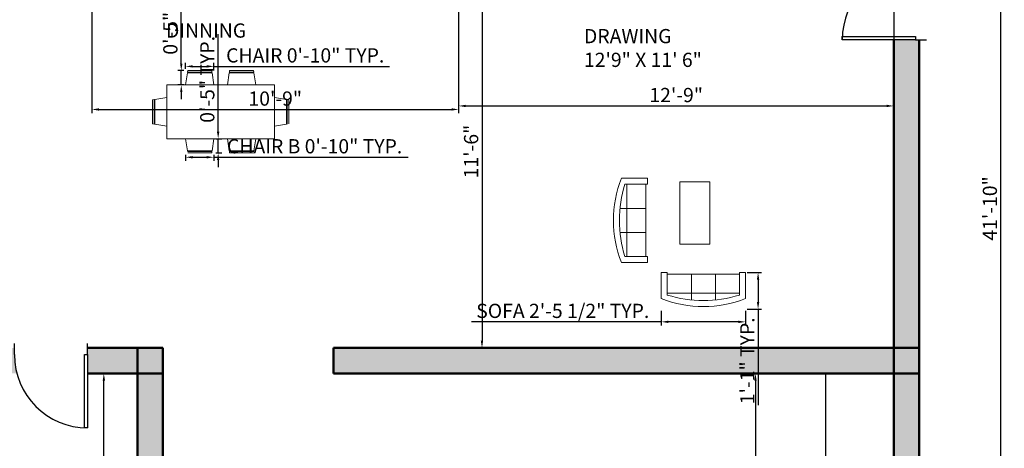
# Model space of a CAD drawing. Units: millimetres. Extents: x 2829 to 4029, y 962 to 1687.
# Tile 3 of 7: x 3053 to 3399, y 1289 to 1440. Entities that reach past the tile are written whole.
import ezdxf

# ---------------------------------------------------------------- set-up
doc = ezdxf.new("R2010")
doc.units = ezdxf.units.MM
for name, color, linetype, lineweight in [('A-ANNO-DIMS', 140, 'Continuous', 18), ('A-AREA-IDEN', 190, 'Continuous', 25), ('A-FLOR-CASE', 90, 'Continuous', 25), ('A-WALL-PATT', 2, 'Continuous', 13), ('doors', 10, 'Continuous', 25), ('furniture', 90, 'Continuous', 18), ('walls', 50, 'Continuous', 50)]:
    doc.layers.add(name, color=color, linetype=linetype, lineweight=lineweight)
doc.styles.get("Standard").update_dxf_attribs({"font": 'arial.ttf'})
doc.dimstyles.new('ISO-25', dxfattribs={"dimtxt": 5, "dimasz": 2.5, "dimexe": 1.25, "dimexo": 0.625, "dimtad": 1, "dimdec": 0, "dimlunit": 3, "dimtxsty": 'Standard', "dimcen": 2.5, "dimadec": 0, "dimazin": 0, "dimtfac": 1, "dimtdec": 0, "dimtmove": 0, "dimatfit": 3, "dimfxl": 1, "dimarcsym": 0})

# ---------------------------------------------------------------- blocks, each defined once
blk = doc.blocks.new('*U2')
for p, q in [((0, 0), (0, -6)), ((40, 0), (40, -6))]:
    blk.add_line(p, q)
blk.add_lwpolyline([(0, 0), (0, 40), (1.75, 40), (1.75, 0)], close=True)
blk.add_arc((0, 0), 40, 0, 90)
blk = doc.blocks.new('Sofa - Roundback 7 ft.')
for p, q in [((-12.00002, -32.4421), (-12.00003, -6.5971)), ((11.99997, -32.4421), (11.99998, -6.5971)), ((-36.000027, -34), (-36.000027, -11.4696)), ((-35.999844, -13.3819), (35.9998, -13.3819)), ((35.99998, -34), (35.99998, -11.4696)), ((-36.000027, -32.4421), (35.99998, -32.4421))]:
    blk.add_line(p, q)
for points in [[(-36.000027, -34), (-42.000027, -34), (-42.000027, -8)], [(41.99998, -8), (41.99998, -34), (35.99998, -34)]]:
    blk.add_lwpolyline(points)
for centre, radius, start, end in [((0, -114.25), 114.25, 68.43141, 111.5686), ((-0.00001, -127.1968), 121.1968, 72.72033, 107.2797)]:
    blk.add_arc(centre, radius, start, end)
blk = doc.blocks.new('*D21')
at = {"layer": 'A-ANNO-DIMS', "color": 0, "lineweight": -2, "transparency": 16777216}
for p, q in [((3080.87, 1315.38), (3083.77, 1315.38)), ((3082.52, 1133.88), (3082.52, 1312.88)), ((3078.75, 1131.38), (3083.77, 1131.38))]:
    blk.add_line(p, q, dxfattribs=at)
at = {"layer": 'A-ANNO-DIMS', "color": 0, "transparency": 16777216}
for points in [[(3082.11, 1312.88), (3082.94, 1312.88), (3082.52, 1315.38)], [(3082.11, 1133.88), (3082.94, 1133.88), (3082.52, 1131.38)]]:
    blk.add_solid(points, dxfattribs=at)
at = {"layer": 'Defpoints', "color": 0, "transparency": 16777216}
for p in [(3080.25, 1315.38), (3082.52, 1315.38), (3078.12, 1131.38)]:
    blk.add_point(p, dxfattribs=at)
at = {"layer": 'A-ANNO-DIMS', "color": 0, "transparency": 16777216, "insert": (3079.34, 1223.38), "char_height": 5, "attachment_point": 5, "rotation": 90}
blk.add_mtext('15\'-4"', dxfattribs=at)
blk = doc.blocks.new('*D25')
at = {"layer": 'A-ANNO-DIMS', "color": 0, "lineweight": -2, "transparency": 16777216}
for p, q in [((3311.7, 1312.88), (3311.7, 1199.88)), ((3312.32, 1315.38), (3312.95, 1315.38)), ((3312.32, 1197.38), (3312.95, 1197.38))]:
    blk.add_line(p, q, dxfattribs=at)
at = {"layer": 'A-ANNO-DIMS', "color": 0, "transparency": 16777216}
for points in [[(3311.28, 1312.88), (3312.11, 1312.88), (3311.7, 1315.38)], [(3311.28, 1199.88), (3312.11, 1199.88), (3311.7, 1197.38)]]:
    blk.add_solid(points, dxfattribs=at)
at = {"layer": 'Defpoints', "color": 0, "transparency": 16777216}
for p in [(3311.7, 1315.38), (3311.7, 1197.38), (3311.7, 1197.38)]:
    blk.add_point(p, dxfattribs=at)
at = {"layer": 'A-ANNO-DIMS', "color": 0, "transparency": 16777216, "insert": (3308.52, 1256.38), "char_height": 5, "attachment_point": 5, "rotation": 90}
blk.add_mtext('9\'-10"', dxfattribs=at)
blk = doc.blocks.new('*D28')
at = {"layer": 'A-ANNO-DIMS', "color": 0, "lineweight": -2, "transparency": 16777216}
for p, q in [((3215.69, 1462.38), (3214.27, 1462.38)), ((3215.52, 1459.88), (3215.52, 1326.88)), ((3215.69, 1324.38), (3214.27, 1324.38))]:
    blk.add_line(p, q, dxfattribs=at)
at = {"layer": 'A-ANNO-DIMS', "color": 0, "transparency": 16777216}
for points in [[(3215.1, 1459.88), (3215.93, 1459.88), (3215.52, 1462.38)], [(3215.1, 1326.88), (3215.93, 1326.88), (3215.52, 1324.38)]]:
    blk.add_solid(points, dxfattribs=at)
at = {"layer": 'Defpoints', "color": 0, "transparency": 16777216}
for p in [(3216.31, 1462.38), (3215.52, 1324.38), (3216.31, 1324.38)]:
    blk.add_point(p, dxfattribs=at)
at = {"layer": 'A-ANNO-DIMS', "color": 0, "transparency": 16777216, "insert": (3212.34, 1393.38), "char_height": 5, "attachment_point": 5, "rotation": 90}
blk.add_mtext('11\'-6"', dxfattribs=at)
blk = doc.blocks.new('*D29')
at = {"layer": 'A-ANNO-DIMS', "color": 0, "lineweight": -2, "transparency": 16777216}
for p, q in [((3207.31, 1461.76), (3207.31, 1408.16)), ((3360.31, 1461.76), (3360.31, 1408.16)), ((3209.81, 1409.41), (3357.81, 1409.41))]:
    blk.add_line(p, q, dxfattribs=at)
at = {"layer": 'A-ANNO-DIMS', "color": 0, "transparency": 16777216}
for points in [[(3209.81, 1409.83), (3209.81, 1408.99), (3207.31, 1409.41)], [(3357.81, 1409.83), (3357.81, 1408.99), (3360.31, 1409.41)]]:
    blk.add_solid(points, dxfattribs=at)
at = {"layer": 'Defpoints', "color": 0, "transparency": 16777216}
for p in [(3207.31, 1462.38), (3360.31, 1462.38), (3360.31, 1409.41)]:
    blk.add_point(p, dxfattribs=at)
at = {"layer": 'A-ANNO-DIMS', "color": 0, "transparency": 16777216, "insert": (3283.81, 1412.59), "char_height": 5, "attachment_point": 5}
blk.add_mtext('12\'-9"', dxfattribs=at)
blk = doc.blocks.new('*D30')
at = {"layer": 'A-ANNO-DIMS', "color": 0, "lineweight": -2, "transparency": 16777216}
for p, q in [((3078.31, 1461.76), (3078.31, 1406.92)), ((3207.31, 1461.76), (3207.31, 1406.92)), ((3080.81, 1408.17), (3204.81, 1408.17))]:
    blk.add_line(p, q, dxfattribs=at)
at = {"layer": 'A-ANNO-DIMS', "color": 0, "transparency": 16777216}
for points in [[(3080.81, 1408.59), (3080.81, 1407.75), (3078.31, 1408.17)], [(3204.81, 1408.59), (3204.81, 1407.75), (3207.31, 1408.17)]]:
    blk.add_solid(points, dxfattribs=at)
at = {"layer": 'Defpoints', "color": 0, "transparency": 16777216}
for p in [(3078.31, 1462.38), (3207.31, 1462.38), (3207.31, 1408.17)]:
    blk.add_point(p, dxfattribs=at)
at = {"layer": 'A-ANNO-DIMS', "color": 0, "transparency": 16777216, "insert": (3142.81, 1411.35), "char_height": 5, "attachment_point": 5}
blk.add_mtext('10\'-9"', dxfattribs=at)
blk = doc.blocks.new('CHAIR-DINING-COMPACT')
for p, q in [((0.66, 4.21), (0, 0)), ((0.66, 4.21), (9.32, 4.21)), ((0.78, 5), (0.7, 4.47)), ((9.28, 4.47), (0.7, 4.47)), ((0.78, 5), (9.2, 5)), ((9.28, 4.47), (9.2, 5)), ((9.98, 0), (9.32, 4.21))]:
    blk.add_line(p, q)
blk = doc.blocks.new('CHAIR-DINING-COMPACT-B')
for p, q in [((0.66, 0.79), (0, 5)), ((9.98, 5), (9.32, 0.79)), ((0.66, 0.79), (9.32, 0.79)), ((9.28, 0.53), (0.7, 0.53)), ((0.78, 0), (9.2, 0)), ((9.28, 0.53), (9.2, 0))]:
    blk.add_line(p, q)
blk = doc.blocks.new('TABLE-COFFEE-RECT')
blk.add_lwpolyline([(0, 0), (10.49, 0), (10.49, 21.96), (0, 21.96)], close=True)
blk = doc.blocks.new('*D65')
at = {"layer": 'A-ANNO-DIMS', "color": 0, "lineweight": -2, "transparency": 16777216}
for p, q in [((3278.58, 1337.35), (3278.58, 1332.28)), ((3308.17, 1337.35), (3308.17, 1332.28)), ((3278.58, 1333.53), (3211.77, 1333.53)), ((3305.67, 1333.53), (3281.08, 1333.53))]:
    blk.add_line(p, q, dxfattribs=at)
at = {"layer": 'A-ANNO-DIMS', "color": 0, "transparency": 16777216}
for points in [[(3281.08, 1333.95), (3281.08, 1333.11), (3278.58, 1333.53)], [(3305.67, 1333.95), (3305.67, 1333.11), (3308.17, 1333.53)]]:
    blk.add_solid(points, dxfattribs=at)
at = {"layer": 'Defpoints', "color": 0, "transparency": 16777216}
for p in [(3278.58, 1337.97), (3308.17, 1337.97), (3278.58, 1333.53)]:
    blk.add_point(p, dxfattribs=at)
at = {"layer": 'A-ANNO-DIMS', "color": 0, "transparency": 16777216, "insert": (3243.92, 1336.74), "char_height": 5, "attachment_point": 5}
blk.add_mtext('SOFA 2\'-5 1/2" TYP.', dxfattribs=at)
blk = doc.blocks.new('*D66')
at = {"layer": 'A-ANNO-DIMS', "color": 0, "lineweight": -2, "transparency": 16777216}
for p, q in [((3308.8, 1350.89), (3313.86, 1350.89)), ((3312.61, 1348.39), (3312.61, 1340.47)), ((3308.8, 1337.97), (3313.86, 1337.97)), ((3312.61, 1337.97), (3312.61, 1304.21))]:
    blk.add_line(p, q, dxfattribs=at)
at = {"layer": 'A-ANNO-DIMS', "color": 0, "transparency": 16777216}
for points in [[(3312.19, 1348.39), (3313.03, 1348.39), (3312.61, 1350.89)], [(3312.19, 1340.47), (3313.03, 1340.47), (3312.61, 1337.97)]]:
    blk.add_solid(points, dxfattribs=at)
at = {"layer": 'Defpoints', "color": 0, "transparency": 16777216}
for p in [(3308.17, 1350.89), (3308.17, 1337.97), (3312.61, 1337.97)]:
    blk.add_point(p, dxfattribs=at)
at = {"layer": 'A-ANNO-DIMS', "color": 0, "transparency": 16777216, "insert": (3309.47, 1319.84), "char_height": 5, "attachment_point": 5, "rotation": 90}
blk.add_mtext('1\'-1" TYP.', dxfattribs=at)
blk = doc.blocks.new('*D79')
at = {"layer": 'A-ANNO-DIMS', "color": 0, "lineweight": -2, "transparency": 16777216}
for p, q in [((3111.25, 1422.43), (3111.25, 1424.56)), ((3113.75, 1423.31), (3118.73, 1423.31)), ((3121.23, 1422.43), (3121.23, 1424.56)), ((3121.23, 1423.31), (3182.96, 1423.31))]:
    blk.add_line(p, q, dxfattribs=at)
at = {"layer": 'A-ANNO-DIMS', "color": 0, "transparency": 16777216}
for points in [[(3113.75, 1423.72), (3113.75, 1422.89), (3111.25, 1423.31)], [(3118.73, 1423.72), (3118.73, 1422.89), (3121.23, 1423.31)]]:
    blk.add_solid(points, dxfattribs=at)
at = {"layer": 'Defpoints', "color": 0, "transparency": 16777216}
for p in [(3121.23, 1423.31), (3111.25, 1421.81), (3121.23, 1421.81)]:
    blk.add_point(p, dxfattribs=at)
at = {"layer": 'A-ANNO-DIMS', "color": 0, "transparency": 16777216, "insert": (3153.35, 1426.52), "char_height": 5, "attachment_point": 5}
blk.add_mtext('CHAIR 0\'-10" TYP.', dxfattribs=at)
blk = doc.blocks.new('*D80')
at = {"layer": 'A-ANNO-DIMS', "color": 0, "lineweight": -2, "transparency": 16777216}
for p, q in [((3109.76, 1424.31), (3109.76, 1458.54)), ((3110.63, 1421.81), (3108.51, 1421.81)), ((3109.76, 1416.81), (3109.76, 1421.81)), ((3110.63, 1416.81), (3108.51, 1416.81)), ((3109.76, 1414.31), (3109.76, 1411.81))]:
    blk.add_line(p, q, dxfattribs=at)
at = {"layer": 'A-ANNO-DIMS', "color": 0, "transparency": 16777216}
for points in [[(3109.34, 1424.31), (3110.17, 1424.31), (3109.76, 1421.81)], [(3109.34, 1414.31), (3110.17, 1414.31), (3109.76, 1416.81)]]:
    blk.add_solid(points, dxfattribs=at)
at = {"layer": 'Defpoints', "color": 0, "transparency": 16777216}
for p in [(3109.76, 1421.81), (3111.25, 1421.81), (3111.25, 1416.81)]:
    blk.add_point(p, dxfattribs=at)
at = {"layer": 'A-ANNO-DIMS', "color": 0, "transparency": 16777216, "insert": (3106.58, 1442.67), "char_height": 5, "attachment_point": 5, "rotation": 90}
blk.add_mtext('0\'-5" TYP.', dxfattribs=at)
blk = doc.blocks.new('*D85')
at = {"layer": 'A-ANNO-DIMS', "color": 0, "lineweight": -2, "transparency": 16777216}
for p, q in [((3111.25, 1392.25), (3111.25, 1390.13)), ((3121.23, 1392.25), (3121.23, 1390.13)), ((3113.75, 1391.38), (3118.73, 1391.38)), ((3121.23, 1391.38), (3189.56, 1391.38))]:
    blk.add_line(p, q, dxfattribs=at)
at = {"layer": 'A-ANNO-DIMS', "color": 0, "transparency": 16777216}
for points in [[(3113.75, 1391.79), (3113.75, 1390.96), (3111.25, 1391.38)], [(3118.73, 1391.79), (3118.73, 1390.96), (3121.23, 1391.38)]]:
    blk.add_solid(points, dxfattribs=at)
at = {"layer": 'Defpoints', "color": 0, "transparency": 16777216}
for p in [(3111.25, 1392.87), (3121.23, 1392.87), (3121.23, 1391.38)]:
    blk.add_point(p, dxfattribs=at)
at = {"layer": 'A-ANNO-DIMS', "color": 0, "transparency": 16777216, "insert": (3156.65, 1394.59), "char_height": 5, "attachment_point": 5}
blk.add_mtext('CHAIR B 0\'-10" TYP.', dxfattribs=at)
blk = doc.blocks.new('*D86')
at = {"layer": 'A-ANNO-DIMS', "color": 0, "lineweight": -2, "transparency": 16777216}
for p, q in [((3122.73, 1400.37), (3122.73, 1434.6)), ((3121.86, 1397.87), (3123.98, 1397.87)), ((3122.73, 1392.87), (3122.73, 1397.87)), ((3121.86, 1392.87), (3123.98, 1392.87)), ((3122.73, 1390.37), (3122.73, 1387.87))]:
    blk.add_line(p, q, dxfattribs=at)
at = {"layer": 'A-ANNO-DIMS', "color": 0, "transparency": 16777216}
for points in [[(3122.31, 1400.37), (3123.15, 1400.37), (3122.73, 1397.87)], [(3122.31, 1390.37), (3123.15, 1390.37), (3122.73, 1392.87)]]:
    blk.add_solid(points, dxfattribs=at)
at = {"layer": 'Defpoints', "color": 0, "transparency": 16777216}
for p in [(3121.23, 1397.87), (3122.73, 1397.87), (3121.23, 1392.87)]:
    blk.add_point(p, dxfattribs=at)
at = {"layer": 'A-ANNO-DIMS', "color": 0, "transparency": 16777216, "insert": (3119.55, 1418.74), "char_height": 5, "attachment_point": 5, "rotation": 90}
blk.add_mtext('0\'-5" TYP.', dxfattribs=at)
blk = doc.blocks.new('*D89')
at = {"layer": 'A-ANNO-DIMS', "color": 0, "lineweight": -2, "transparency": 16777216}
for p, q in [((2853.31, 1314.76), (2853.31, 1094.98)), ((3369.31, 1121.76), (3369.31, 1094.98)), ((2855.81, 1096.23), (3366.81, 1096.23))]:
    blk.add_line(p, q, dxfattribs=at)
at = {"layer": 'A-ANNO-DIMS', "color": 0, "transparency": 16777216}
for points in [[(2855.81, 1096.65), (2855.81, 1095.81), (2853.31, 1096.23)], [(3366.81, 1096.65), (3366.81, 1095.81), (3369.31, 1096.23)]]:
    blk.add_solid(points, dxfattribs=at)
at = {"layer": 'Defpoints', "color": 0, "transparency": 16777216}
for p in [(2853.31, 1315.38), (3369.31, 1122.38), (3369.31, 1096.23)]:
    blk.add_point(p, dxfattribs=at)
at = {"layer": 'A-ANNO-DIMS', "color": 0, "transparency": 16777216, "insert": (3111.31, 1099.41), "char_height": 5, "attachment_point": 5}
blk.add_mtext('43\'-0"', dxfattribs=at)
blk = doc.blocks.new('*D90')
at = {"layer": 'A-ANNO-DIMS', "color": 0, "lineweight": -2, "transparency": 16777216}
for p, q in [((3369.94, 1624.38), (3399.21, 1624.38)), ((3397.96, 1124.88), (3397.96, 1621.88)), ((3369.94, 1122.38), (3399.21, 1122.38))]:
    blk.add_line(p, q, dxfattribs=at)
at = {"layer": 'A-ANNO-DIMS', "color": 0, "transparency": 16777216}
for points in [[(3397.54, 1621.88), (3398.38, 1621.88), (3397.96, 1624.38)], [(3397.54, 1124.88), (3398.38, 1124.88), (3397.96, 1122.38)]]:
    blk.add_solid(points, dxfattribs=at)
at = {"layer": 'Defpoints', "color": 0, "transparency": 16777216}
for p in [(3369.31, 1624.38), (3397.96, 1624.38), (3369.31, 1122.38)]:
    blk.add_point(p, dxfattribs=at)
at = {"layer": 'A-ANNO-DIMS', "color": 0, "transparency": 16777216, "insert": (3394.78, 1373.38), "char_height": 5, "attachment_point": 5, "rotation": 90}
blk.add_mtext('41\'-10"', dxfattribs=at)

msp = doc.modelspace()

# ---------------------------------------------------------------- hatches: boundary and pattern name
at = {"layer": 'A-WALL-PATT'}
h = msp.add_hatch(color=256, dxfattribs=at)
h.dxf.hatch_style = 1
h.paths.add_polyline_path([(2969.05, 1624.38), (2937.31, 1624.38), (2937.31, 1615.38), (2969.05, 1615.38)])
h.paths.add_polyline_path([(2937.31, 1624.38), (2928.31, 1624.38), (2928.31, 1615.38), (2937.31, 1615.38)])
h.paths.add_polyline_path([(2937.31, 1615.38), (2928.31, 1615.38), (2928.31, 1471.38), (2937.31, 1471.38)])
h.paths.add_polyline_path([(3069.31, 1624.38), (3011.61, 1624.38), (3011.61, 1615.38), (3069.31, 1615.38)])
h.paths.add_polyline_path([(3078.31, 1624.38), (3069.31, 1624.38), (3069.31, 1615.38), (3078.31, 1615.38)])
h.paths.add_polyline_path([(3078.31, 1615.38), (3069.31, 1615.38), (3069.31, 1581.62), (3069.43, 1581.62), (3078.31, 1581.62)])
h.paths.add_polyline_path([(3078.31, 1566.24, -0.131652), (3069.43, 1563.86), (3069.31, 1563.86), (3069.31, 1519.38), (3078.31, 1519.38)])
h.paths.add_polyline_path([(3078.31, 1519.38), (3069.31, 1519.38), (3069.31, 1510.38), (3078.31, 1510.38)])
h.paths.add_polyline_path([(3138.31, 1519.38), (3078.31, 1519.38), (3078.31, 1510.38), (3138.31, 1510.38)])
h.paths.add_polyline_path([(3147.31, 1519.38), (3138.31, 1519.38), (3138.31, 1510.38), (3147.31, 1510.38)])
h.paths.add_polyline_path([(3147.31, 1615.38), (3138.31, 1615.38), (3138.31, 1519.38), (3147.31, 1519.38)])
h.paths.add_polyline_path([(3147.31, 1624.38), (3138.31, 1624.38), (3138.31, 1615.38), (3147.31, 1615.38)])
h.paths.add_polyline_path([(3138.31, 1624.38), (3116.25, 1624.38), (3116.25, 1615.38), (3138.31, 1615.38)])
h.paths.add_polyline_path([(3096.9, 1624.38), (3078.31, 1624.38), (3078.31, 1615.38), (3096.9, 1615.38)])
h.paths.add_polyline_path([(3167.88, 1624.38), (3147.31, 1624.38), (3147.31, 1615.38), (3167.88, 1615.38)])
h.paths.add_polyline_path([(3207.31, 1624.38), (3186.66, 1624.38), (3186.66, 1615.38), (3207.31, 1615.38)])
h.paths.add_polyline_path([(3216.31, 1624.38), (3207.31, 1624.38), (3207.31, 1615.38), (3216.31, 1615.38)])
h.paths.add_polyline_path([(3216.31, 1615.38), (3207.31, 1615.38), (3207.31, 1585.36), (3216.31, 1585.36)])
h.paths.add_polyline_path([(3216.31, 1567.6), (3216.21, 1567.6, -0.131958), (3207.31, 1569.99), (3207.31, 1519.38), (3216.31, 1519.38)])
h.paths.add_polyline_path([(3216.31, 1519.38), (3207.31, 1519.38), (3207.31, 1510.38), (3216.31, 1510.38)])
h.paths.add_polyline_path([(3207.31, 1519.38), (3147.31, 1519.38), (3147.31, 1510.38), (3207.31, 1510.38)])
h.paths.add_polyline_path([(3269.97, 1624.38), (3216.31, 1624.38), (3216.31, 1615.38), (3269.97, 1615.38)])
h.paths.add_polyline_path([(3360.31, 1624.38), (3310.37, 1624.38), (3310.37, 1615.38), (3360.31, 1615.38)])
h.paths.add_polyline_path([(3369.31, 1624.38), (3360.31, 1624.38), (3360.31, 1615.38), (3369.31, 1615.38)])
h.paths.add_polyline_path([(3369.31, 1615.38), (3360.31, 1615.38), (3360.31, 1471.38), (3369.31, 1471.38)])
h.paths.add_polyline_path([(3360.31, 1471.38), (3216.31, 1471.38), (3216.31, 1462.38), (3360.31, 1462.38)])
h.paths.add_polyline_path([(3216.31, 1471.38), (3207.31, 1471.38), (3207.31, 1462.38), (3216.31, 1462.38)])
h.paths.add_polyline_path([(3216.31, 1479.42, -0.089587), (3207.31, 1477.74), (3207.31, 1471.38), (3216.31, 1471.38)])
h.paths.add_polyline_path([(3216.31, 1510.38), (3207.31, 1510.38), (3207.31, 1503.49), (3216.31, 1503.49)])
h.paths.add_polyline_path([(3369.31, 1471.38), (3360.31, 1471.38), (3360.31, 1462.38), (3369.31, 1462.38)])
h.paths.add_polyline_path([(3360.31, 1324.38), (3163.31, 1324.38), (3163.31, 1315.38), (3360.31, 1315.38)])
h.paths.add_polyline_path([(3369.31, 1324.38), (3360.31, 1324.38), (3360.31, 1315.38), (3369.31, 1315.38)])
h.paths.add_polyline_path([(3028.89, 1471.38), (2937.31, 1471.38), (2937.31, 1462.38), (3028.89, 1462.38), (3028.89, 1465.26)])
h.paths.add_polyline_path([(2937.31, 1471.38), (2928.31, 1471.38), (2928.31, 1462.38), (2937.31, 1462.38)])
h.paths.add_polyline_path([(2928.31, 1471.38), (2862.31, 1471.38), (2862.31, 1462.38), (2928.31, 1462.38)])
h.paths.add_polyline_path([(2862.31, 1462.38), (2853.31, 1462.38), (2853.31, 1324.38), (2862.31, 1324.38)])
h.paths.add_polyline_path([(2862.31, 1471.38), (2853.31, 1471.38), (2853.31, 1462.38), (2862.31, 1462.38)])
h.paths.add_polyline_path([(2928.31, 1324.38), (2862.31, 1324.38), (2862.31, 1315.38), (2928.31, 1315.38)])
h.paths.add_polyline_path([(2862.31, 1324.38), (2853.31, 1324.38), (2853.31, 1315.38), (2862.31, 1315.38)])
h.paths.add_polyline_path([(3051.08, 1322.02), (3051.08, 1324.38), (2937.31, 1324.38), (2937.31, 1315.38), (3051.95, 1315.38, -0.065323)])
h.paths.add_polyline_path([(2937.31, 1324.38), (2928.31, 1324.38), (2928.31, 1315.38), (2937.31, 1315.38)])
h.paths.add_polyline_path([(3103.31, 1315.38), (3094.31, 1315.38), (3094.31, 1248.38), (3103.31, 1248.38)])
h.paths.add_polyline_path([(3103.31, 1324.38), (3094.31, 1324.38), (3094.31, 1315.38), (3103.31, 1315.38)])
h.paths.add_polyline_path([(3094.31, 1324.38), (3076.83, 1324.38), (3076.83, 1322.02), (3076.83, 1315.38), (3094.31, 1315.38)])
h.paths.add_polyline_path([(3078.31, 1510.38), (3069.31, 1510.38), (3069.31, 1471.38), (3078.31, 1471.38)])
h.paths.add_polyline_path([(3078.31, 1471.38), (3069.31, 1471.38), (3069.31, 1462.38), (3078.31, 1462.38)])
h.paths.add_polyline_path([(3069.31, 1471.38), (3053.91, 1471.38, -0.060076), (3054.65, 1465.26), (3054.65, 1462.38), (3069.31, 1462.38)])
h.paths.add_polyline_path([(2937.31, 1315.38), (2928.31, 1315.38), (2928.31, 1131.38), (2937.31, 1131.38)])
h.paths.add_polyline_path([(2937.31, 1131.38), (2928.31, 1131.38), (2928.31, 1122.38), (2937.31, 1122.38)])
h.paths.add_polyline_path([(2978.9, 1131.38), (2937.31, 1131.38), (2937.31, 1122.38), (2978.9, 1122.38)])
h.paths.add_polyline_path([(3094.31, 1131.38), (3017.24, 1131.38), (3017.24, 1122.38), (3094.31, 1122.38)])
h.paths.add_polyline_path([(3103.31, 1131.38), (3094.31, 1131.38), (3094.31, 1122.38), (3103.31, 1122.38)])
h.paths.add_polyline_path([(3103.31, 1179.58, -0.112378), (3095.63, 1177.83), (3094.31, 1177.83), (3094.31, 1131.38), (3103.31, 1131.38)])
h.paths.add_polyline_path([(3103.31, 1239.38), (3094.31, 1239.38), (3094.31, 1195.59), (3095.63, 1195.59), (3103.31, 1195.59)])
h.paths.add_polyline_path([(3103.31, 1248.38), (3094.31, 1248.38), (3094.31, 1239.38), (3103.31, 1239.38)])
h.paths.add_polyline_path([(3163.31, 1248.38), (3103.31, 1248.38), (3103.31, 1239.38), (3163.31, 1239.38)])
h.paths.add_polyline_path([(3172.31, 1248.38), (3163.31, 1248.38), (3163.31, 1239.38), (3172.31, 1239.38)])
h.paths.add_polyline_path([(3172.31, 1239.38), (3163.31, 1239.38), (3163.31, 1197.38), (3172.31, 1197.38)])
h.paths.add_polyline_path([(3172.31, 1197.38), (3163.31, 1197.38), (3163.31, 1188.38), (3172.31, 1188.38)])
h.paths.add_polyline_path([(3172.31, 1188.38), (3163.31, 1188.38), (3163.31, 1131.38), (3172.31, 1131.38)])
h.paths.add_polyline_path([(3172.31, 1131.38), (3163.31, 1131.38), (3163.31, 1122.38), (3172.31, 1122.38)])
h.paths.add_polyline_path([(3163.31, 1131.38), (3143.05, 1131.38), (3143.05, 1122.38), (3163.31, 1122.38)])
h.paths.add_polyline_path([(3123.82, 1131.38), (3103.31, 1131.38), (3103.31, 1122.38), (3123.82, 1122.38)])
h.paths.add_polyline_path([(3273.8, 1131.38), (3172.31, 1131.38), (3172.31, 1122.38), (3273.8, 1122.38)])
h.paths.add_polyline_path([(3360.31, 1131.38), (3293.49, 1131.38), (3293.49, 1122.38), (3360.31, 1122.38)])
h.paths.add_polyline_path([(3369.31, 1131.38), (3360.31, 1131.38), (3360.31, 1122.38), (3369.31, 1122.38)])
h.paths.add_polyline_path([(3369.31, 1188.38), (3360.31, 1188.38), (3360.31, 1131.38), (3369.31, 1131.38)])
h.paths.add_polyline_path([(3369.31, 1197.38), (3360.31, 1197.38), (3360.31, 1188.38), (3369.31, 1188.38)])
h.paths.add_polyline_path([(3360.31, 1197.38), (3252.19, 1197.38), (3252.19, 1188.38), (3360.31, 1188.38)])
h.paths.add_polyline_path([(3234.43, 1197.38), (3172.31, 1197.38), (3172.31, 1188.38), (3237.05, 1188.38, -0.134312)])
h.paths.add_polyline_path([(3369.31, 1315.38), (3360.31, 1315.38), (3360.31, 1197.38), (3369.31, 1197.38)])
edge = h.paths.add_edge_path()
edge.add_arc((3367.95, 1432.65), 25.75, 90, 107.2357)
edge.add_line((3360.31, 1457.25), (3360.31, 1462.38))
edge.add_line((3360.31, 1462.38), (3369.31, 1462.38))
edge.add_line((3369.31, 1462.38), (3369.31, 1458.41))
edge.add_line((3369.31, 1458.41), (3367.95, 1458.41))
h.paths.add_polyline_path([(3369.31, 1432.65), (3360.31, 1432.65), (3360.31, 1324.38), (3369.31, 1324.38)])

# ---------------------------------------------------------------- linework, layer by layer
at = {"layer": 'A-FLOR-CASE'}
for p, q in [((3360.31, 1315.38), (3336.31, 1315.38)), ((3336.31, 1315.38), (3336.31, 1221.14))]:
    msp.add_line(p, q, dxfattribs=at)
at = {"layer": 'furniture'}
for p, q in [((3142.55, 1416.81), (3104.67, 1416.81)), ((3104.67, 1416.81), (3104.67, 1397.87)), ((3142.55, 1397.87), (3142.55, 1416.81)), ((3146.76, 1411.67), (3142.55, 1412.33)), ((3146.76, 1411.67), (3146.76, 1403.01)), ((3147.02, 1403.05), (3147.02, 1411.63)), ((3147.55, 1411.55), (3147.55, 1403.13)), ((3142.55, 1402.35), (3146.76, 1403.01)), ((3104.67, 1397.87), (3142.55, 1397.87))]:
    msp.add_line(p, q, dxfattribs=at)
at = {"layer": 'walls'}
for p, q in [((3360.31, 1432.65), (3360.31, 1122.38)), ((3369.31, 1432.65), (3369.31, 1122.38)), ((3076.83, 1324.38), (3103.31, 1324.38)), ((3094.31, 1324.38), (3094.31, 1195.59)), ((3103.31, 1324.38), (3103.31, 1195.59)), ((3163.31, 1324.38), (3369.31, 1324.38)), ((3163.31, 1324.38), (3163.31, 1315.38)), ((3076.83, 1315.38), (3103.31, 1315.38)), ((3163.31, 1315.38), (3369.31, 1315.38))]:
    msp.add_line(p, q, dxfattribs=at)

# ---------------------------------------------------------------- block references
at = {"layer": 'doors', "xscale": 0.6438655246665308, "yscale": 0.6438655246665308, "zscale": 0.6438655246665308}
for p, rotation in [((3367.95, 1432.65), 90), ((3076.83, 1322.02), 180)]:
    msp.add_blockref('*U2', p, dxfattribs=dict(at, rotation=rotation))
at = {"layer": 'furniture'}
for name, p in [('CHAIR-DINING-COMPACT', (3111.25, 1416.81)), ('CHAIR-DINING-COMPACT', (3125.98, 1416.81)), ('CHAIR-DINING-COMPACT-B', (3111.25, 1392.87)), ('TABLE-COFFEE-RECT', (3285.15, 1360.83))]:
    msp.add_blockref(name, p, dxfattribs=at)
at = {"layer": 'furniture', "extrusion": (0, 0, -1), "zscale": -1}
for name, p, rotation in [('CHAIR-DINING-COMPACT', (-3104.67, 1412.33), 269.9999718792713), ('CHAIR-DINING-COMPACT-B', (-3135.96, 1392.87), 359.9942656820082)]:
    msp.add_blockref(name, p, dxfattribs=dict(at, rotation=rotation))
at = {"layer": 'furniture', "xscale": 0.3523046889690534, "yscale": 0.3523046889690534, "zscale": 0.3523046889690534}
for p, rotation in [((3261.74, 1369.19), 89.99999999999999), ((3293.38, 1338.91), 180)]:
    msp.add_blockref('Sofa - Roundback 7 ft.', p, dxfattribs=dict(at, rotation=rotation))

# ---------------------------------------------------------------- texts
at = {"layer": 'A-AREA-IDEN', "char_height": 5, "attachment_point": 1}
for s, width, insert in [('DINNING ', 44.3787, (3104.4, 1438.41)), ('DRAWING \\P12\'9" X 11\' 6"', 54.0277, (3251.38, 1436.44))]:
    msp.add_mtext_dynamic_manual_height_columns(s, width=width, gutter_width=12.5, heights=[0], dxfattribs=dict(at, insert=insert))

# ---------------------------------------------------------------- dimensions: what is measured, and where the dimension line sits
at = {"layer": 'A-ANNO-DIMS'}
for base, p1, p2, override, picture, middle in [((3397.96, 1624.38), (3369.31, 1122.38), (3369.31, 1624.38), {"dimdec": 1, "dimlfac": 1, "dimrnd": 0, "dimzin": 1, "dimdsep": 46, "dimlunit": 4, "dimfrac": 2}, '*D90', (3394.78, 1373.38)), ((3215.52, 1324.38), (3216.31, 1462.38), (3216.31, 1324.38), {"dimclrd": 0, "dimclre": 0, "dimclrt": 0}, '*D28', (3212.34, 1393.38)), ((3082.52, 1315.38), (3078.12, 1131.38), (3080.25, 1315.38), {"dimclrd": 0, "dimclre": 0, "dimclrt": 0}, '*D21', (3079.34, 1223.38)), ((3311.7, 1197.38), (3311.7, 1315.38), (3311.7, 1197.38), {"dimclrd": 0, "dimclre": 0, "dimclrt": 0}, '*D25', (3308.52, 1256.38))]:
    dim = msp.add_linear_dim(base=base, p1=p1, p2=p2, angle=90, dimstyle='ISO-25', override=override, dxfattribs=at)
    dim.commit()
    dim.dimension.update_dxf_attribs({"geometry": picture, "text_midpoint": middle})
for base, p1, p2, override, picture, middle in [((3207.31, 1408.17), (3078.31, 1462.38), (3207.31, 1462.38), {"dimclrd": 0, "dimclre": 0, "dimclrt": 0}, '*D30', (3142.81, 1411.35)), ((3360.31, 1409.41), (3207.31, 1462.38), (3360.31, 1462.38), {"dimclrd": 0, "dimclre": 0, "dimclrt": 0}, '*D29', (3283.81, 1412.59)), ((3369.31, 1096.23), (2853.31, 1315.38), (3369.31, 1122.38), {"dimdec": 1, "dimlfac": 1, "dimrnd": 0, "dimzin": 1, "dimdsep": 46, "dimlunit": 4, "dimfrac": 2}, '*D89', (3111.31, 1099.41))]:
    dim = msp.add_linear_dim(base=base, p1=p1, p2=p2, dimstyle='ISO-25', override=override, dxfattribs=at)
    dim.commit()
    dim.dimension.update_dxf_attribs({"geometry": picture, "text_midpoint": middle})
for base, p1, p2, angle, text, picture, middle in [((3109.76, 1421.81), (3111.25, 1416.81), (3111.25, 1421.81), 90, '<> TYP.', '*D80', (3106.58, 1442.67)), ((3122.73, 1397.87), (3121.23, 1392.87), (3121.23, 1397.87), 90, '<> TYP.', '*D86', (3119.55, 1418.74)), ((3278.58, 1333.53), (3308.17, 1337.97), (3278.58, 1337.97), 180, 'SOFA <> TYP.', '*D65', (3243.92, 1336.74)), ((3312.61, 1337.97), (3308.17, 1350.89), (3308.17, 1337.97), 270, '<> TYP.', '*D66', (3309.47, 1319.84))]:
    dim = msp.add_linear_dim(base=base, p1=p1, p2=p2, angle=angle, text=text, dimstyle='ISO-25', override={"dimdec": 1, "dimlfac": 1, "dimrnd": 0, "dimzin": 1, "dimdsep": 46, "dimlunit": 4, "dimfrac": 2}, dxfattribs=at)
    dim.commit()
    dim.dimension.update_dxf_attribs({"geometry": picture, "text_midpoint": middle})
for base, p1, p2, text, picture, middle in [((3121.23, 1423.31), (3111.25, 1421.81), (3121.23, 1421.81), 'CHAIR <> TYP.', '*D79', (3153.35, 1426.52)), ((3121.23, 1391.38), (3111.25, 1392.87), (3121.23, 1392.87), 'CHAIR B <> TYP.', '*D85', (3156.65, 1394.59))]:
    dim = msp.add_linear_dim(base=base, p1=p1, p2=p2, text=text, dimstyle='ISO-25', override={"dimdec": 1, "dimlfac": 1, "dimrnd": 0, "dimzin": 1, "dimdsep": 46, "dimlunit": 4, "dimfrac": 2}, dxfattribs=at)
    dim.commit()
    dim.dimension.update_dxf_attribs({"geometry": picture, "text_midpoint": middle})

doc.saveas('drawing.dxf')
